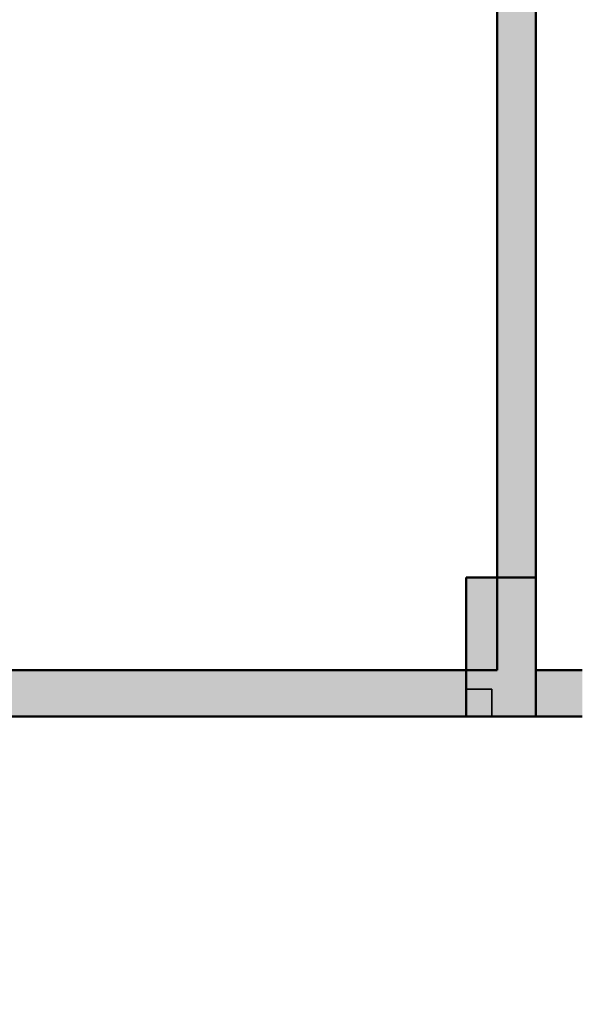
# Model space of a CAD drawing. Units: inches. Extents: x -7 to 1228, y -146 to 1091.
# Tile 47 of 88: x 169 to 242, y 531 to 658. Entities that reach past the tile are written whole.
import ezdxf

# ---------------------------------------------------------------- set-up
doc = ezdxf.new("R2010")
doc.units = ezdxf.units.IN
for name, color, linetype, lineweight in [('A-COLS', 6, 'Continuous', 35), ('A-WALL', 7, 'Continuous', 50), ('A-WALL-PATT', 251, 'Continuous', 13)]:
    doc.layers.add(name, color=color, linetype=linetype, lineweight=lineweight)

msp = doc.modelspace()

# ---------------------------------------------------------------- hatches: boundary and pattern name
at = {"layer": 'A-COLS'}
h = msp.add_hatch(color=256, dxfattribs=at)
h.dxf.hatch_style = 1
h.paths.add_polyline_path([(227, 571.55), (230.29, 571.55), (230.29, 568), (236, 568), (236, 586), (227, 586)])
h = msp.add_hatch(color=256, dxfattribs=at)
h.dxf.hatch_style = 1
h.paths.add_polyline_path([(227, 571.55), (227, 568), (230.29, 568), (230.29, 571.55)])
at = {"layer": 'A-WALL-PATT'}
h = msp.add_hatch(color=256, dxfattribs=at)
h.dxf.hatch_style = 1
h.paths.add_polyline_path([(69, 568), (60, 568), (60, 493), (63.29, 493), (69, 493)])
h.paths.add_polyline_path([(69, 662.41), (60, 662.41), (60, 586), (69, 586)], flags=17)
h.paths.add_polyline_path([(69, 723), (184, 723), (184, 734), (179, 734), (179, 728), (69, 728), (69, 741.62), (60, 741.62), (60, 698.41), (69, 698.41)], flags=17)
h.paths.add_polyline_path([(69, 782), (231, 782), (231, 728), (231, 723), (231, 586), (236, 586), (236, 787), (69, 787), (69, 800.13), (60, 800.13), (60, 765.62), (69, 765.62)])
h.paths.add_polyline_path([(184, 842), (189, 842), (189, 848), (173, 848), (173, 842), (179, 842), (179, 787), (184, 787)])
h.paths.add_polyline_path([(118.22, 69), (69, 69), (69, 60), (118.22, 60)])
h.paths.add_polyline_path([(227, 69), (154.22, 69), (154.22, 60), (227, 60)])
h.paths.add_polyline_path([(236, 60), (232.71, 60), (227, 60), (227, 36), (236, 36)])
h.paths.add_polyline_path([(389, 60), (380, 60), (380, 36), (389, 36)])
h.paths.add_polyline_path([(384, 181), (380, 181), (380, 115), (380, 78), (384, 78)])
h.paths.add_polyline_path([(380, 115), (334.55, 115), (334.55, 109), (380, 109)])
h.paths.add_polyline_path([(274.55, 115), (236, 115), (236, 201), (232.71, 201), (231, 201), (231, 78), (236, 78), (236, 109), (274.55, 109)])
h.paths.add_polyline_path([(69, 123), (60, 123), (60, 78), (69, 78)])
h.paths.add_polyline_path([(69, 201), (60, 201), (60, 159), (69, 159)])
h.paths.add_polyline_path([(143, 219), (69, 219), (69, 213), (143, 213)], flags=17)
h.paths.add_polyline_path([(189, 219), (184, 219), (184, 274), (231, 274), (231, 219), (236, 219), (236, 279), (184, 279), (184, 297), (179, 297), (179, 279), (69, 279), (69, 290.91), (60, 290.91), (60, 262.18), (69, 262.18), (69, 274), (179, 274), (179, 219), (173, 219), (173, 213), (189, 213)])
h.paths.add_polyline_path([(69, 238.18), (60, 238.18), (60, 219), (69, 219)], flags=17)
h.paths.add_polyline_path([(69, 333), (60, 333), (60, 314.91), (69, 314.91), (69, 316.96)])
h.paths.add_polyline_path([(190, 338), (184, 338), (69, 338), (69, 333), (179, 333), (179, 327), (184, 327), (184, 333.02), (190, 333.05)])
h.paths.add_polyline_path([(69, 386.81), (60, 386.81), (60, 351), (69, 351)])
h.paths.add_polyline_path([(69, 475), (60, 475), (60, 422.81), (69, 422.81)])
h.paths.add_polyline_path([(236, 475), (231, 475), (231, 351.24), (236, 351.24)])
h.paths.add_polyline_path([(384, 475), (380, 475), (380, 362), (384, 362)])
h.paths.add_polyline_path([(547, 307), (439, 307), (439, 356), (445, 356), (445, 362), (433, 362), (433, 307), (380, 307), (380, 244), (380, 241), (384, 241), (384, 301), (433, 301), (433, 277), (439, 277), (439, 301), (547, 301)])
h.paths.add_polyline_path([(547, 241), (439, 241), (439, 247), (433, 247), (433, 235), (547, 235)])
h.paths.add_polyline_path([(450, 69), (440.29, 69), (424.89, 69), (389, 69), (389, 60), (450, 60)])
h.paths.add_polyline_path([(547, 69), (486, 69), (486, 60), (547, 60)])
h.paths.add_polyline_path([(556, 148.27), (547, 148.27), (547, 78), (556, 78)])
h.paths.add_polyline_path([(556, 223), (547, 223), (547, 195), (547, 184.27), (556, 184.27)])
h.paths.add_polyline_path([(556, 311.19), (547, 311.19), (547, 273.08), (556, 273.08)])
h.paths.add_polyline_path([(556, 344), (552.71, 344), (547, 344), (547, 335.19), (556, 335.19)])
h.paths.add_polyline_path([(556, 249.08), (547, 249.08), (547, 241), (556, 241)])
h.paths.add_polyline_path([(547, 362), (475, 362), (475, 356), (547, 356)], flags=0)
h.paths.add_polyline_path([(556, 399.62), (547, 399.62), (547, 362), (556, 362)])
h.paths.add_polyline_path([(556, 475), (547, 475), (547, 435.62), (556, 435.62)])
h.paths.add_polyline_path([(547, 493), (389, 493), (389, 487), (547, 487)])
h.paths.add_polyline_path([(380, 493), (278, 493), (278, 487), (380, 487)])
h.paths.add_polyline_path([(227, 493), (69, 493), (69, 487), (227, 487)])
h.paths.add_polyline_path([(643, 122.44), (634, 122.44), (634, 78), (643, 78)])
h.paths.add_polyline_path([(702.5, 69), (692.79, 69), (677.39, 69), (643, 69), (643, 60), (702.5, 60)])
h.paths.add_polyline_path([(798, 69), (738.5, 69), (738.5, 60), (798, 60)])
h.paths.add_polyline_path([(807, 60), (803.71, 60), (798, 60), (798, 36), (807, 36)])
h.paths.add_polyline_path([(807, 109), (846.75, 109), (846.75, 115), (807, 115), (807, 159), (802, 159), (802, 78), (807, 78)])
h.paths.add_polyline_path([(807, 201), (802, 201), (802, 195), (807, 195)])
h.paths.add_polyline_path([(643, 201), (634, 201), (634, 158.44), (643, 158.44)])
h.paths.add_polyline_path([(756, 225), (751, 225), (751, 219), (643, 219), (643, 213), (756, 213)])
h.paths.add_polyline_path([(643, 240.85), (634, 240.85), (634, 219), (643, 219)])
h.paths.add_polyline_path([(643, 274), (643, 288.63), (634, 288.63), (634, 264.85), (643, 264.85)])
h.paths.add_polyline_path([(802, 279), (756, 279), (756, 297), (751, 297), (751, 279), (643, 279), (643, 274), (751, 274), (751, 255), (756, 255), (756, 274), (802, 274)])
h.paths.add_polyline_path([(807, 333), (803.71, 333), (802, 333), (802, 279), (802, 274), (802, 219), (807, 219)])
h.paths.add_polyline_path([(956, 182), (951, 182), (951, 115), (906.75, 115), (906.75, 109), (951, 109), (951, 78), (956, 78)])
h.paths.add_polyline_path([(960, 60), (951, 60), (951, 36), (960, 36)])
h.paths.add_polyline_path([(1021, 69), (1005.78, 69), (960, 69), (960, 60), (1021, 60)])
h.paths.add_polyline_path([(956, 224), (951, 224), (951, 218), (956, 218)])
h.paths.add_polyline_path([(956, 302), (1004, 302), (1004, 278), (1010, 278), (1010, 302), (1118, 302), (1118, 290.81), (1127, 290.81), (1127, 326.97), (1118, 326.97), (1118, 320.97), (1118, 307), (1010, 307), (1010, 356), (1016, 356), (1016, 362), (1004, 362), (1004, 307), (951, 307), (951, 244), (951, 242), (954.29, 242), (956, 242)])
h.paths.add_polyline_path([(643, 333), (634, 333), (634, 312.63), (643, 312.63), (643, 316.96)])
h.paths.add_polyline_path([(756, 338), (643, 338), (643, 333), (751, 333), (751, 327), (756, 327)])
h.paths.add_polyline_path([(643, 388), (634, 388), (634, 351), (643, 351)])
h.paths.add_polyline_path([(807, 357), (802, 357), (802, 351), (807, 351)])
h.paths.add_polyline_path([(807, 475), (802, 475), (802, 393), (807, 393)])
h.paths.add_polyline_path([(643, 475), (634, 475), (634, 424), (643, 424)])
h.paths.add_polyline_path([(798, 493), (643, 493), (643, 487), (798, 487)])
h.paths.add_polyline_path([(634, 493), (556, 493), (556, 487), (634, 487)])
h.paths.add_polyline_path([(813, 493), (807, 493), (807, 487), (813, 487)])
h.paths.add_polyline_path([(951, 493), (849, 493), (849, 487), (951, 487)])
h.paths.add_polyline_path([(956, 484), (951, 484), (951, 374), (956, 374)])
h.paths.add_polyline_path([(1109, 493), (969, 493), (969, 487), (1109, 487)])
h.paths.add_polyline_path([(1127, 484), (1118, 484), (1118, 450.64), (1127, 450.64)])
h.paths.add_polyline_path([(1127, 414.64), (1118, 414.64), (1118, 365), (1127, 365)])
h.paths.add_polyline_path([(1109, 362), (1046, 362), (1046, 356), (1109, 356)], flags=17)
h.paths.add_polyline_path([(1127, 356), (1123.45, 356), (1118, 356), (1118, 350.97), (1127, 350.97)], flags=0)
h.paths.add_polyline_path([(1127, 266.81), (1118, 266.81), (1118, 262.36), (1118, 242), (1127, 242)], flags=17)
h.paths.add_polyline_path([(1118, 242), (1010, 242), (1010, 248), (1004, 248), (1004, 237), (1118, 237)])
h.paths.add_polyline_path([(1127, 224), (1118, 224), (1118, 170), (1127, 170)])
h.paths.add_polyline_path([(1127, 134), (1118, 134), (1118, 78), (1127, 78)])
h.paths.add_polyline_path([(1118, 69), (1057, 69), (1057, 60), (1118, 60)])
h.paths.add_polyline_path([(227, 571.55), (227, 574), (69, 574), (69, 568), (227, 568)])
h.paths.add_polyline_path([(380, 571.55), (380, 574), (278, 574), (278, 568), (380, 568)])
h.paths.add_polyline_path([(242, 574), (236, 574), (236, 568), (242, 568)])
h.paths.add_polyline_path([(547, 571.55), (547, 574), (389, 574), (389, 568), (547, 568)])
h.paths.add_polyline_path([(384, 733), (380, 733), (380, 586), (384, 586)])
h.paths.add_polyline_path([(556, 646), (634, 646), (634, 655), (547, 655), (547, 586), (556, 586)])
h.paths.add_polyline_path([(634, 574), (556, 574), (556, 568), (634, 568)])
h.paths.add_polyline_path([(643, 655), (634, 655), (634, 586), (643, 586)])
h.paths.add_polyline_path([(798, 574), (643, 574), (643, 568), (798, 568)])
h.paths.add_polyline_path([(643, 663.85), (634, 663.85), (634, 655), (643, 655)])
h.paths.add_polyline_path([(556, 676.97), (547, 676.97), (547, 655), (556, 655)])
h.paths.add_polyline_path([(556, 733), (547, 733), (547, 712.97), (556, 712.97)])
h.paths.add_polyline_path([(643, 710), (634, 710), (634, 699.85), (643, 699.85)])
h.paths.add_polyline_path([(807, 668), (802, 668), (802, 586), (807, 586)])
h.paths.add_polyline_path([(951, 574), (849, 574), (849, 568), (951, 568)])
h.paths.add_polyline_path([(956, 691), (951, 691), (951, 577), (956, 577)])
h.paths.add_polyline_path([(1109, 574), (969, 574), (969, 568), (1109, 568)])
h.paths.add_polyline_path([(1127, 643.4), (1118, 643.4), (1118, 577), (1127, 577)])
h.paths.add_polyline_path([(1127, 568), (1123.45, 568), (1118, 568), (1118, 493), (1127, 493)])
h.paths.add_polyline_path([(1127, 733), (1118, 733), (1118, 679.4), (1127, 679.4)])
h.paths.add_polyline_path([(1127, 777.35), (1118, 777.35), (1118, 770.04), (1118, 751), (1127, 751)], flags=17)
h.paths.add_polyline_path([(1118, 751), (1010, 751), (1010, 757), (1004, 757), (1004, 745), (1118, 745)])
h.paths.add_polyline_path([(956, 811), (1004, 811), (1004, 787), (1010, 787), (1010, 811), (1017.87, 811), (1017.87, 811.63, -0.414214), (1018.25, 812), (1031.98, 812, -0.414214), (1032.35, 811.63), (1032.35, 811), (1118, 811), (1118, 801.35), (1127, 801.35), (1127, 834.69), (1118, 834.69), (1118, 830.24), (1118, 817), (1010, 817), (1010, 866), (1016, 866), (1016, 872), (1004, 872), (1004, 817), (956, 817), (956, 866), (951, 866), (951, 751), (954.29, 751), (956, 751)])
h.paths.add_polyline_path([(1118, 872), (1046, 872), (1046, 866), (1118, 866)], flags=17)
h.paths.add_polyline_path([(1127, 924.71), (1118, 924.71), (1118, 884), (1127, 884)])
h.paths.add_polyline_path([(1127, 866), (1123.71, 866), (1118, 866), (1118, 858.69), (1127, 858.69)], flags=17)
h.paths.add_polyline_path([(956, 983), (951, 983), (951, 952), (807, 952), (807, 983), (802, 983), (802, 902), (807, 902), (807, 946), (951, 946), (951, 884), (956, 884)])
h.paths.add_polyline_path([(807, 842), (802, 842), (802, 787), (756, 787), (756, 806), (751, 806), (751, 787), (643, 787), (643, 782), (751, 782), (751, 764), (756, 764), (756, 782), (802, 782), (802, 728), (807, 728)])
h.paths.add_polyline_path([(756, 848), (643, 848), (643, 842), (751, 842), (751, 836), (756, 836)])
h.paths.add_polyline_path([(756, 734), (751, 734), (751, 728), (643, 728), (643, 723), (756, 723)])
h.paths.add_polyline_path([(643, 749.79), (634, 749.79), (634, 728), (637.29, 728), (643, 728)])
h.paths.add_polyline_path([(643, 805.41), (634, 805.41), (634, 773.79), (643, 773.79)])
h.paths.add_polyline_path([(643, 896.66), (634, 896.66), (634, 860), (637.29, 860), (643, 860)])
h.paths.add_polyline_path([(643, 842), (634, 842), (634, 829.41), (643, 829.41)])
h.paths.add_polyline_path([(643, 983), (634, 983), (634, 932.66), (643, 932.66)])
h.paths.add_polyline_path([(1127, 983), (1118, 983), (1118, 960.71), (1127, 960.71)])
h.paths.add_polyline_path([(1118, 1001), (1077.53, 1001), (1077.53, 992), (1118, 992)])
h.paths.add_polyline_path([(1041.53, 1001), (960, 1001), (960, 992), (1041.53, 992)])
h.paths.add_polyline_path([(960, 1025), (951, 1025), (951, 1001), (954.29, 1001), (960, 1001)])
h.paths.add_polyline_path([(807, 1025), (798, 1025), (798, 1001), (807, 1001)])
h.paths.add_polyline_path([(798, 1001), (738.5, 1001), (738.5, 992), (798, 992)])
h.paths.add_polyline_path([(702.5, 1001), (643, 1001), (643, 992), (702.5, 992)])
h.paths.add_polyline_path([(547, 1001), (499.11, 1001), (499.11, 992), (547, 992)])
h.paths.add_polyline_path([(463.11, 1001), (389, 1001), (389, 992), (463.11, 992)])
h.paths.add_polyline_path([(389, 1025), (380, 1025), (380, 1022), (380, 1001), (383.29, 1001), (389, 1001)])
h.paths.add_polyline_path([(236, 1025), (227, 1025), (227, 1001), (236, 1001)])
h.paths.add_polyline_path([(236, 983), (231, 983), (231, 860), (236, 860)])
h.paths.add_polyline_path([(274.55, 952), (236, 952), (236, 946), (274.55, 946)])
h.paths.add_polyline_path([(380, 952), (334.55, 952), (334.55, 946), (380, 946)])
h.paths.add_polyline_path([(384, 983), (380, 983), (380, 884), (383.29, 884), (384, 884)])
h.paths.add_polyline_path([(227, 1001), (155.01, 1001), (155.01, 992), (162.87, 992), (227, 992)])
h.paths.add_polyline_path([(119.01, 1001), (69, 1001), (69, 992), (119.01, 992)])
h.paths.add_polyline_path([(69, 983), (60, 983), (60, 922.99), (69, 922.99)])
h.paths.add_polyline_path([(69, 886.99), (60, 886.99), (60, 860), (63.29, 860), (69, 860)])
h.paths.add_polyline_path([(143, 848), (69, 848), (69, 842), (143, 842)])

# ---------------------------------------------------------------- linework, layer by layer
at = {"layer": 'A-COLS'}
msp.add_lwpolyline([(227, 568), (230.29, 568), (230.29, 571.55), (227, 571.55)], close=True, dxfattribs=at)
at = {"layer": 'A-WALL'}
for p, q in [((236, 787), (236, 574)), ((231, 723), (231, 574)), ((236, 586), (227, 586)), ((227, 586), (227, 568)), ((236, 568), (236, 586)), ((231, 574), (69, 574)), ((242, 574), (236, 574)), ((231, 568), (60, 568)), ((227, 568), (236, 568)), ((242, 568), (236, 568))]:
    msp.add_line(p, q, dxfattribs=at)

doc.saveas('drawing.dxf')
